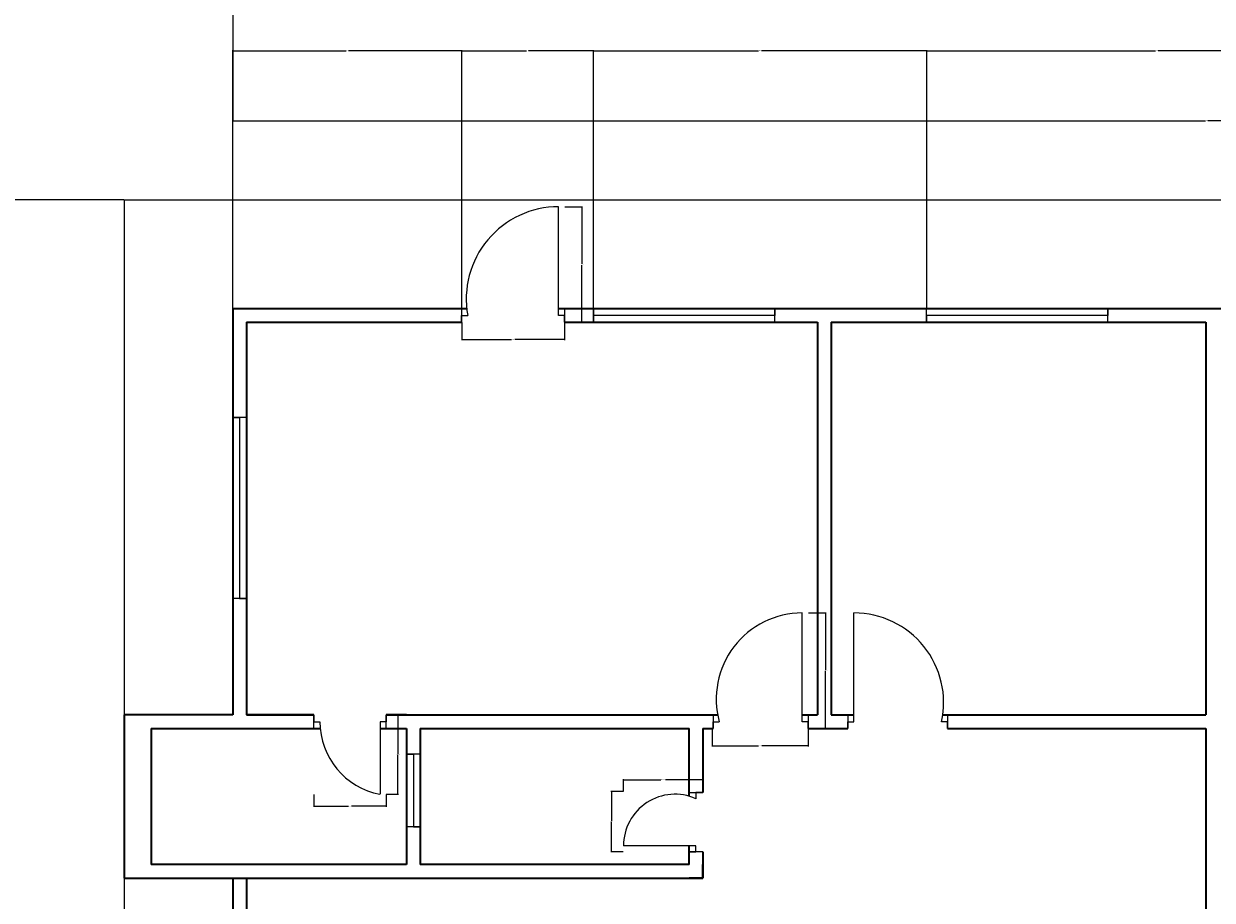
# Model space of a CAD drawing. Units: inches. Extents: x 1520 to 3401, y 1570 to 3432.
# Tile 12 of 15: x 2435 to 2828, y 2501 to 2791. Entities that reach past the tile are written whole.
import ezdxf

# ---------------------------------------------------------------- set-up
doc = ezdxf.new("R2010")
doc.units = ezdxf.units.IN
for name, color, linetype, lineweight in [('A-ANNO-DIMS', 2, 'Continuous', 18), ('A-DOOR', 3, 'Continuous', 18), ('A-FLOR-EDGE', 7, 'Continuous', 25), ('A-GLAZ', 4, 'Continuous', 18), ('A-WALL', 7, 'Continuous', 35)]:
    doc.layers.add(name, color=color, linetype=linetype, lineweight=lineweight)
doc.styles.get("Standard").update_dxf_attribs({"font": 'arial.ttf'})
doc.dimstyles.get("Standard").update_dxf_attribs({"dimtxt": 0.18, "dimasz": 0.18, "dimexe": 0.18, "dimexo": 0.0625, "dimgap": 0.09, "dimtad": 0, "dimtih": 1, "dimtoh": 1, "dimdec": 4, "dimzin": 0, "dimdsep": 46, "dimtxsty": 'Standard', "dimcen": 0.09, "dimadec": 0, "dimazin": 0, "dimtfac": 1, "dimtdec": 4, "dimtofl": 0, "dimtmove": 0, "dimatfit": 3, "dimfxl": 1, "dimtolj": 1, "dimtzin": 0, "dimarcsym": 0})

# ---------------------------------------------------------------- blocks, each defined once
blk = doc.blocks.new('DOOR-SWING-24-01')
for p, q in [((21.75, 19.61), (26.25, 19.61)), ((26.25, 19.61), (24, 19.61)), ((24, 19.61), (24, 17.61)), ((24, 2), (0, 2)), ((24, 0), (24, 2)), ((26.25, 0), (21.75, 0)), ((21.75, 0), (24, 0))]:
    blk.add_line(p, q)
blk.add_arc((17.08, 2), 17.08, 66.0978, 180)
blk = doc.blocks.new('DOOR-SWING-24-02')
for p, q in [((0, 21.75), (0, 26.25)), ((0, 26.25), (0, 24)), ((0, 24), (2, 24)), ((23.89, 24), (21.89, 24)), ((21.89, 24), (21.89, 0)), ((23.89, 21.75), (23.89, 26.25)), ((23.89, 26.25), (23.89, 24))]:
    blk.add_line(p, q)
blk.add_arc((26.42, 24), 24.42, 180, 259.3013)
blk = doc.blocks.new('DOOR-SWING-36-03')
for p, q in [((29.45, 2.25), (29.45, 38.25)), ((0, 4.5), (0, 0)), ((31.45, 4.5), (31.45, 0)), ((0, 0), (0, 2.25)), ((0, 2.25), (2, 2.25)), ((31.45, 2.25), (29.45, 2.25)), ((31.45, 0), (31.45, 2.25))]:
    blk.add_line(p, q)
blk.add_arc((29.45, 9.79), 28.46, 90, 195.3561)
blk = doc.blocks.new('DOOR-SWING-36-04')
for p, q in [((2, 2.25), (2, 38.25)), ((0, 4.5), (0, 0)), ((32.99, 4.5), (32.99, 0)), ((0, 0), (0, 2.25)), ((0, 2.25), (2, 2.25)), ((32.99, 2.25), (30.99, 2.25)), ((32.99, 0), (32.99, 2.25))]:
    blk.add_line(p, q)
blk.add_arc((2, 8.58), 29.67, 347.6919, 90)
blk = doc.blocks.new('DOOR-SWING-36-22')
for p, q in [((32.08, 2.25), (32.08, 38.25)), ((0, 4.5), (0, 0)), ((34.08, 4.5), (34.08, 0)), ((0, 0), (0, 2.25)), ((0, 2.25), (2, 2.25)), ((34.08, 2.25), (32.08, 2.25)), ((34.08, 0), (34.08, 2.25))]:
    blk.add_line(p, q)
blk.add_arc((32.08, 7.69), 30.56, 90, 190.2449)
blk = doc.blocks.new('WIN-PLAN-24-01')
for p, q in [((0, 4.5), (0, 0)), ((24, 2.25), (24, 4.5)), ((24, 4.5), (24, 0)), ((0, 0), (0, 2.25)), ((0, 2.25), (24, 2.25))]:
    blk.add_line(p, q)
blk = doc.blocks.new('WIN-PLAN-60-02')
for p, q in [((4.5, 60), (0, 60)), ((0, 60), (2.25, 60)), ((2.25, 60), (2.25, 0)), ((4.5, 0), (0, 0)), ((2.25, 0), (4.5, 0))]:
    blk.add_line(p, q)
blk = doc.blocks.new('WIN-PLAN-60-03')
for p, q in [((0, 2.25), (0, 4.5)), ((0, 4.5), (0, 0)), ((60, 0), (60, 4.5)), ((60, 4.5), (60, 2.25)), ((60, 2.25), (0, 2.25))]:
    blk.add_line(p, q)
blk = doc.blocks.new('*D81')
at = {"layer": 'A-ANNO-DIMS', "color": 0, "lineweight": -2, "transparency": 16777216}
for p, q in [((2633.15, 2537.36), (2633.15, 2541.41)), ((2633.33, 2541.23), (2645.48, 2541.23)), ((2659.22, 2541.23), (2647.06, 2541.23)), ((2659.4, 2537.36), (2659.4, 2541.41))]:
    blk.add_line(p, q, dxfattribs=at)
at = {"layer": 'A-ANNO-DIMS', "color": 0, "transparency": 16777216}
for points in [[(2633.33, 2541.26), (2633.33, 2541.2), (2633.15, 2541.23)], [(2659.22, 2541.26), (2659.22, 2541.2), (2659.4, 2541.23)]]:
    blk.add_solid(points, dxfattribs=at)
at = {"layer": 'Defpoints', "color": 0, "transparency": 16777216}
for p in [(2659.4, 2541.23), (2633.15, 2537.3), (2659.4, 2537.3)]:
    blk.add_point(p, dxfattribs=at)
at = {"layer": 'A-ANNO-DIMS', "color": 0, "transparency": 16777216, "insert": (2646.27, 2541.23), "char_height": 0.18, "attachment_point": 5}
blk.add_mtext('\\A1;D01 26 TYP.', dxfattribs=at)
blk = doc.blocks.new('*D82')
at = {"layer": 'A-ANNO-DIMS', "color": 0, "lineweight": -2, "transparency": 16777216}
for p, q in [((2633.09, 2537.3), (2629.03, 2537.3)), ((2629.21, 2537.12), (2629.21, 2527.5)), ((2629.21, 2517.52), (2629.21, 2527.14)), ((2633.09, 2517.34), (2629.03, 2517.34))]:
    blk.add_line(p, q, dxfattribs=at)
at = {"layer": 'A-ANNO-DIMS', "color": 0, "transparency": 16777216}
for points in [[(2629.18, 2537.12), (2629.24, 2537.12), (2629.21, 2537.3)], [(2629.18, 2517.52), (2629.24, 2517.52), (2629.21, 2517.34)]]:
    blk.add_solid(points, dxfattribs=at)
at = {"layer": 'Defpoints', "color": 0, "transparency": 16777216}
for p in [(2629.21, 2537.3), (2633.15, 2537.3), (2633.15, 2517.34)]:
    blk.add_point(p, dxfattribs=at)
at = {"layer": 'A-ANNO-DIMS', "color": 0, "transparency": 16777216, "insert": (2629.21, 2527.32), "char_height": 0.18, "attachment_point": 5}
blk.add_mtext('\\A1;20 TYP.', dxfattribs=at)
blk = doc.blocks.new('*D83')
at = {"layer": 'A-ANNO-DIMS', "color": 0, "lineweight": -2, "transparency": 16777216}
for p, q in [((2554.66, 2562.68), (2558.71, 2562.68)), ((2558.53, 2562.5), (2558.53, 2549.74)), ((2558.53, 2536.61), (2558.53, 2549.37)), ((2554.66, 2536.43), (2558.71, 2536.43))]:
    blk.add_line(p, q, dxfattribs=at)
at = {"layer": 'A-ANNO-DIMS', "color": 0, "transparency": 16777216}
for points in [[(2558.5, 2562.5), (2558.56, 2562.5), (2558.53, 2562.68)], [(2558.5, 2536.61), (2558.56, 2536.61), (2558.53, 2536.43)]]:
    blk.add_solid(points, dxfattribs=at)
at = {"layer": 'Defpoints', "color": 0, "transparency": 16777216}
for p in [(2554.6, 2562.68), (2558.53, 2562.68), (2554.6, 2536.43)]:
    blk.add_point(p, dxfattribs=at)
at = {"layer": 'A-ANNO-DIMS', "color": 0, "transparency": 16777216, "insert": (2558.53, 2549.55), "char_height": 0.18, "attachment_point": 5}
blk.add_mtext('\\A1;D02 26 TYP.', dxfattribs=at)
blk = doc.blocks.new('*D84')
at = {"layer": 'A-ANNO-DIMS', "color": 0, "lineweight": -2, "transparency": 16777216}
for p, q in [((2530.7, 2536.37), (2530.7, 2532.31)), ((2554.6, 2536.37), (2554.6, 2532.31)), ((2530.88, 2532.49), (2542.12, 2532.49)), ((2554.42, 2532.49), (2543.18, 2532.49))]:
    blk.add_line(p, q, dxfattribs=at)
at = {"layer": 'A-ANNO-DIMS', "color": 0, "transparency": 16777216}
for points in [[(2530.88, 2532.52), (2530.88, 2532.46), (2530.7, 2532.49)], [(2554.42, 2532.52), (2554.42, 2532.46), (2554.6, 2532.49)]]:
    blk.add_solid(points, dxfattribs=at)
at = {"layer": 'Defpoints', "color": 0, "transparency": 16777216}
for p in [(2530.7, 2536.43), (2554.6, 2536.43), (2554.6, 2532.49)]:
    blk.add_point(p, dxfattribs=at)
at = {"layer": 'A-ANNO-DIMS', "color": 0, "transparency": 16777216, "insert": (2542.65, 2532.49), "char_height": 0.18, "attachment_point": 5}
blk.add_mtext('\\A1;24 TYP.', dxfattribs=at)
blk = doc.blocks.new('*D85')
at = {"layer": 'A-ANNO-DIMS', "color": 0, "lineweight": -2, "transparency": 16777216}
for p, q in [((2694.38, 2596.43), (2700.24, 2596.43)), ((2700.06, 2596.25), (2700.06, 2577.49)), ((2700.06, 2558.36), (2700.06, 2577.12)), ((2694.38, 2558.18), (2700.24, 2558.18))]:
    blk.add_line(p, q, dxfattribs=at)
at = {"layer": 'A-ANNO-DIMS', "color": 0, "transparency": 16777216}
for points in [[(2700.03, 2596.25), (2700.09, 2596.25), (2700.06, 2596.43)], [(2700.03, 2558.36), (2700.09, 2558.36), (2700.06, 2558.18)]]:
    blk.add_solid(points, dxfattribs=at)
at = {"layer": 'Defpoints', "color": 0, "transparency": 16777216}
for p in [(2694.32, 2596.43), (2700.06, 2596.43), (2694.32, 2558.18)]:
    blk.add_point(p, dxfattribs=at)
at = {"layer": 'A-ANNO-DIMS', "color": 0, "transparency": 16777216, "insert": (2700.06, 2577.3), "char_height": 0.18, "attachment_point": 5}
blk.add_mtext('\\A1;D03 38 TYP.', dxfattribs=at)
blk = doc.blocks.new('*D86')
at = {"layer": 'A-ANNO-DIMS', "color": 0, "lineweight": -2, "transparency": 16777216}
for p, q in [((2662.52, 2558.12), (2662.52, 2552.26)), ((2694.32, 2558.12), (2694.32, 2552.26)), ((2662.7, 2552.44), (2677.89, 2552.44)), ((2694.14, 2552.44), (2678.95, 2552.44))]:
    blk.add_line(p, q, dxfattribs=at)
at = {"layer": 'A-ANNO-DIMS', "color": 0, "transparency": 16777216}
for points in [[(2662.7, 2552.47), (2662.7, 2552.41), (2662.52, 2552.44)], [(2694.14, 2552.47), (2694.14, 2552.41), (2694.32, 2552.44)]]:
    blk.add_solid(points, dxfattribs=at)
at = {"layer": 'Defpoints', "color": 0, "transparency": 16777216}
for p in [(2662.52, 2558.18), (2694.32, 2558.18), (2694.32, 2552.44)]:
    blk.add_point(p, dxfattribs=at)
at = {"layer": 'A-ANNO-DIMS', "color": 0, "transparency": 16777216, "insert": (2678.42, 2552.44), "char_height": 0.18, "attachment_point": 5}
blk.add_mtext('\\A1;32 TYP.', dxfattribs=at)
blk = doc.blocks.new('*D123')
at = {"layer": 'A-ANNO-DIMS', "color": 0, "lineweight": -2, "transparency": 16777216}
for p, q in [((2613.76, 2730.93), (2619.61, 2730.93)), ((2619.43, 2730.75), (2619.43, 2711.99)), ((2619.43, 2692.86), (2619.43, 2711.62)), ((2613.76, 2692.68), (2619.61, 2692.68))]:
    blk.add_line(p, q, dxfattribs=at)
at = {"layer": 'A-ANNO-DIMS', "color": 0, "transparency": 16777216}
for points in [[(2619.4, 2730.75), (2619.46, 2730.75), (2619.43, 2730.93)], [(2619.4, 2692.86), (2619.46, 2692.86), (2619.43, 2692.68)]]:
    blk.add_solid(points, dxfattribs=at)
at = {"layer": 'Defpoints', "color": 0, "transparency": 16777216}
for p in [(2613.69, 2730.93), (2619.43, 2730.93), (2613.69, 2692.68)]:
    blk.add_point(p, dxfattribs=at)
at = {"layer": 'A-ANNO-DIMS', "color": 0, "transparency": 16777216, "insert": (2619.43, 2711.8), "char_height": 0.18, "attachment_point": 5}
blk.add_mtext('\\A1;D22 38 TYP.', dxfattribs=at)
blk = doc.blocks.new('*D124')
at = {"layer": 'A-ANNO-DIMS', "color": 0, "lineweight": -2, "transparency": 16777216}
for p, q in [((2579.62, 2692.62), (2579.62, 2686.76)), ((2613.69, 2692.62), (2613.69, 2686.76)), ((2579.8, 2686.94), (2596.13, 2686.94)), ((2613.51, 2686.94), (2597.18, 2686.94))]:
    blk.add_line(p, q, dxfattribs=at)
at = {"layer": 'A-ANNO-DIMS', "color": 0, "transparency": 16777216}
for points in [[(2579.8, 2686.97), (2579.8, 2686.91), (2579.62, 2686.94)], [(2613.51, 2686.97), (2613.51, 2686.91), (2613.69, 2686.94)]]:
    blk.add_solid(points, dxfattribs=at)
at = {"layer": 'Defpoints', "color": 0, "transparency": 16777216}
for p in [(2579.62, 2692.68), (2613.69, 2692.68), (2613.69, 2686.94)]:
    blk.add_point(p, dxfattribs=at)
at = {"layer": 'A-ANNO-DIMS', "color": 0, "transparency": 16777216, "insert": (2596.65, 2686.94), "char_height": 0.18, "attachment_point": 5}
blk.add_mtext('\\A1;34 TYP.', dxfattribs=at)
blk = doc.blocks.new('*D192')
at = {"layer": 'A-ANNO-DIMS', "color": 0, "lineweight": -2, "transparency": 16777216}
for p, q in [((2467.84, 2733.18), (2386.32, 2733.18)), ((2386.5, 2733), (2386.5, 2244.61)), ((2386.5, 1755.86), (2386.5, 2244.25)), ((2503.84, 1755.68), (2386.32, 1755.68))]:
    blk.add_line(p, q, dxfattribs=at)
at = {"layer": 'A-ANNO-DIMS', "color": 0, "transparency": 16777216}
for points in [[(2386.47, 2733), (2386.53, 2733), (2386.5, 2733.18)], [(2386.47, 1755.86), (2386.53, 1755.86), (2386.5, 1755.68)]]:
    blk.add_solid(points, dxfattribs=at)
at = {"layer": 'Defpoints', "color": 0, "transparency": 16777216}
for p in [(2467.9, 2733.18), (2386.5, 1755.68), (2503.9, 1755.68)]:
    blk.add_point(p, dxfattribs=at)
at = {"layer": 'A-ANNO-DIMS', "color": 0, "transparency": 16777216, "insert": (2386.5, 2244.43), "char_height": 0.18, "attachment_point": 5}
blk.add_mtext('\\A1;977.5', dxfattribs=at)
blk = doc.blocks.new('*D202')
at = {"layer": 'A-ANNO-DIMS', "color": 0, "lineweight": -2, "transparency": 16777216}
for p, q in [((2503.9, 2697.24), (2503.9, 2782.76)), ((2504.08, 2782.58), (2541.37, 2782.58)), ((2579.44, 2782.58), (2542.15, 2782.58)), ((2579.62, 2692.74), (2579.62, 2782.76))]:
    blk.add_line(p, q, dxfattribs=at)
at = {"layer": 'A-ANNO-DIMS', "color": 0, "transparency": 16777216}
for points in [[(2504.08, 2782.61), (2504.08, 2782.55), (2503.9, 2782.58)], [(2579.44, 2782.61), (2579.44, 2782.55), (2579.62, 2782.58)]]:
    blk.add_solid(points, dxfattribs=at)
at = {"layer": 'Defpoints', "color": 0, "transparency": 16777216}
for p in [(2579.62, 2782.58), (2503.9, 2697.18), (2579.62, 2692.68)]:
    blk.add_point(p, dxfattribs=at)
at = {"layer": 'A-ANNO-DIMS', "color": 0, "transparency": 16777216, "insert": (2541.76, 2782.58), "char_height": 0.18, "attachment_point": 5}
blk.add_mtext('\\A1;75.72', dxfattribs=at)
blk = doc.blocks.new('*D203')
at = {"layer": 'A-ANNO-DIMS', "color": 0, "lineweight": -2, "transparency": 16777216}
for p, q in [((2579.62, 2692.74), (2579.62, 2782.76)), ((2579.8, 2782.58), (2601.09, 2782.58)), ((2623.04, 2782.58), (2601.74, 2782.58)), ((2623.22, 2692.74), (2623.22, 2782.76))]:
    blk.add_line(p, q, dxfattribs=at)
at = {"layer": 'A-ANNO-DIMS', "color": 0, "transparency": 16777216}
for points in [[(2579.8, 2782.61), (2579.8, 2782.55), (2579.62, 2782.58)], [(2623.04, 2782.61), (2623.04, 2782.55), (2623.22, 2782.58)]]:
    blk.add_solid(points, dxfattribs=at)
at = {"layer": 'Defpoints', "color": 0, "transparency": 16777216}
for p in [(2623.22, 2782.58), (2579.62, 2692.68), (2623.22, 2692.68)]:
    blk.add_point(p, dxfattribs=at)
at = {"layer": 'A-ANNO-DIMS', "color": 0, "transparency": 16777216, "insert": (2601.42, 2782.58), "char_height": 0.18, "attachment_point": 5}
blk.add_mtext('\\A1;43.6', dxfattribs=at)
blk = doc.blocks.new('*D204')
at = {"layer": 'A-ANNO-DIMS', "color": 0, "lineweight": -2, "transparency": 16777216}
for p, q in [((2623.22, 2692.74), (2623.22, 2782.76)), ((2623.4, 2782.58), (2677.9, 2782.58)), ((2733.32, 2782.58), (2678.81, 2782.58)), ((2733.5, 2697.24), (2733.5, 2782.76))]:
    blk.add_line(p, q, dxfattribs=at)
at = {"layer": 'A-ANNO-DIMS', "color": 0, "transparency": 16777216}
for points in [[(2623.4, 2782.61), (2623.4, 2782.55), (2623.22, 2782.58)], [(2733.32, 2782.61), (2733.32, 2782.55), (2733.5, 2782.58)]]:
    blk.add_solid(points, dxfattribs=at)
at = {"layer": 'Defpoints', "color": 0, "transparency": 16777216}
for p in [(2733.5, 2782.58), (2733.5, 2697.18), (2623.22, 2692.68)]:
    blk.add_point(p, dxfattribs=at)
at = {"layer": 'A-ANNO-DIMS', "color": 0, "transparency": 16777216, "insert": (2678.36, 2782.58), "char_height": 0.18, "attachment_point": 5}
blk.add_mtext('\\A1;110.28', dxfattribs=at)
blk = doc.blocks.new('*D205')
at = {"layer": 'A-ANNO-DIMS', "color": 0, "lineweight": -2, "transparency": 16777216}
for p, q in [((2733.5, 2697.24), (2733.5, 2782.76)), ((2733.68, 2782.58), (2809.22, 2782.58)), ((2885.68, 2782.58), (2810.13, 2782.58)), ((2885.86, 2692.74), (2885.86, 2782.76))]:
    blk.add_line(p, q, dxfattribs=at)
at = {"layer": 'A-ANNO-DIMS', "color": 0, "transparency": 16777216}
for points in [[(2733.68, 2782.61), (2733.68, 2782.55), (2733.5, 2782.58)], [(2885.68, 2782.61), (2885.68, 2782.55), (2885.86, 2782.58)]]:
    blk.add_solid(points, dxfattribs=at)
at = {"layer": 'Defpoints', "color": 0, "transparency": 16777216}
for p in [(2885.86, 2782.58), (2733.5, 2697.18), (2885.86, 2692.68)]:
    blk.add_point(p, dxfattribs=at)
at = {"layer": 'A-ANNO-DIMS', "color": 0, "transparency": 16777216, "insert": (2809.68, 2782.58), "char_height": 0.18, "attachment_point": 5}
blk.add_mtext('\\A1;152.37', dxfattribs=at)
blk = doc.blocks.new('*D224')
at = {"layer": 'A-ANNO-DIMS', "color": 0, "lineweight": -2, "transparency": 16777216}
for p, q in [((2503.9, 2875.57), (2503.9, 2759.2)), ((3148.4, 2875.57), (3148.4, 2759.2)), ((2504.08, 2759.38), (2825.75, 2759.38)), ((3148.22, 2759.38), (2826.54, 2759.38))]:
    blk.add_line(p, q, dxfattribs=at)
at = {"layer": 'A-ANNO-DIMS', "color": 0, "transparency": 16777216}
for points in [[(2504.08, 2759.41), (2504.08, 2759.35), (2503.9, 2759.38)], [(3148.22, 2759.41), (3148.22, 2759.35), (3148.4, 2759.38)]]:
    blk.add_solid(points, dxfattribs=at)
at = {"layer": 'Defpoints', "color": 0, "transparency": 16777216}
for p in [(2503.9, 2875.63), (3148.4, 2875.63), (3148.4, 2759.38)]:
    blk.add_point(p, dxfattribs=at)
at = {"layer": 'A-ANNO-DIMS', "color": 0, "transparency": 16777216, "insert": (2826.15, 2759.38), "char_height": 0.18, "attachment_point": 5}
blk.add_mtext('\\A1;644.5', dxfattribs=at)

msp = doc.modelspace()

# ---------------------------------------------------------------- linework, layer by layer
at = {"layer": 'A-FLOR-EDGE'}
for q in [(2467.8987, 1791.6786), (3184.3987, 2733.1786)]:
    msp.add_line((2467.8987, 2733.1786), q, dxfattribs=at)
at = {"layer": 'A-WALL'}
for p, q in [((2503.8987, 2697.1786), (2503.8987, 2562.6786)), ((2503.8987, 2697.1786), (2503.8987, 2562.6786)), ((2503.8987, 2697.1786), (2581.2953, 2697.1786)), ((2611.6928, 2697.1786), (2887.6429, 2697.1786)), ((2508.3987, 2692.6786), (2508.3987, 2562.6786)), ((2508.3987, 2692.6786), (2579.616, 2692.6786)), ((2613.6928, 2692.6786), (2697.3987, 2692.6786)), ((2697.3987, 2692.6786), (2697.3987, 2562.6786)), ((2701.8987, 2692.6786), (2701.8987, 2562.6786)), ((2701.8987, 2692.6786), (2825.8987, 2692.6786)), ((2825.8987, 2692.6786), (2825.8987, 2562.6786)), ((2503.8987, 2562.6786), (2467.8987, 2562.6786)), ((2467.8987, 2562.6786), (2467.8987, 2508.6786)), ((2508.3987, 2562.6786), (2530.705, 2562.6786)), ((2530.705, 2562.6786), (2508.3987, 2562.6786)), ((2554.5952, 2562.6786), (2664.3512, 2562.6786)), ((2561.3987, 2562.6786), (2554.5952, 2562.6786)), ((2692.3184, 2562.6786), (2697.3987, 2562.6786)), ((2701.8987, 2562.6786), (2709.4502, 2562.6786)), ((2738.8433, 2562.6786), (2825.8987, 2562.6786)), ((2476.8987, 2558.1786), (2532.8088, 2558.1786)), ((2476.8987, 2558.1786), (2476.8987, 2513.1786)), ((2552.5952, 2558.1786), (2561.3987, 2558.1786)), ((2561.3987, 2558.1786), (2561.3987, 2513.1786)), ((2565.8987, 2558.1786), (2565.8987, 2513.1786)), ((2565.8987, 2558.1786), (2654.8987, 2558.1786)), ((2654.8987, 2535.7697), (2654.8987, 2558.1786)), ((2659.3987, 2558.1786), (2662.8719, 2558.1786)), ((2659.3987, 2558.1786), (2659.3987, 2536.9559)), ((2694.3184, 2558.1786), (2707.4502, 2558.1786)), ((2740.4425, 2558.1786), (2825.8987, 2558.1786)), ((2825.8987, 2558.1786), (2825.8987, 2343.1786)), ((2654.8987, 2513.1786), (2654.8987, 2519.341)), ((2659.3987, 2517.341), (2659.3987, 2508.6786)), ((2561.3987, 2513.1786), (2476.8987, 2513.1786)), ((2654.8987, 2513.1786), (2565.8987, 2513.1786)), ((2659.3987, 2508.6786), (2659.3987, 2513.1786)), ((2467.8987, 2508.6786), (2565.8987, 2508.6786)), ((2503.8987, 2508.6786), (2503.8987, 2425.0977)), ((2503.8987, 2508.6786), (2503.8987, 2425.0977)), ((2508.3987, 2508.6786), (2508.3987, 2423.0977)), ((2508.3987, 2508.6786), (2631.3987, 2508.6786)), ((2565.8987, 2508.6786), (2631.3987, 2508.6786)), ((2631.3987, 2508.6786), (2635.8987, 2508.6786)), ((2635.8987, 2508.6786), (2654.8987, 2508.6786)), ((2659.3987, 2508.6786), (2654.8987, 2508.6786)), ((2654.8987, 2508.6786), (2659.3987, 2508.6786))]:
    msp.add_line(p, q, dxfattribs=at)

# ---------------------------------------------------------------- block references
at = {"layer": 'A-DOOR'}
for name, p in [('DOOR-SWING-36-22', (2579.6158, 2692.679)), ('DOOR-SWING-36-03', (2662.8718, 2558.179)), ('DOOR-SWING-36-04', (2707.4498, 2558.179)), ('DOOR-SWING-24-02', (2530.7048, 2536.429)), ('DOOR-SWING-24-01', (2633.1488, 2517.341))]:
    msp.add_blockref(name, p, dxfattribs=at)
at = {"layer": 'A-GLAZ'}
for name, p in [('WIN-PLAN-60-03', (2623.2164, 2692.679)), ('WIN-PLAN-60-02', (2503.8988, 2601.185))]:
    msp.add_blockref(name, p, dxfattribs=at)
at = {"layer": 'A-GLAZ', "rotation": 270}
for name, p in [('WIN-PLAN-60-02', (2733.496, 2697.1785)), ('WIN-PLAN-24-01', (2561.399, 2549.6622))]:
    msp.add_blockref(name, p, dxfattribs=at)

# ---------------------------------------------------------------- dimensions: what is measured, and where the dimension line sits
at = {"layer": 'A-ANNO-DIMS'}
for base, p1, p2, override, picture, middle in [((3148.3987, 2759.3805), (2503.8987, 2875.633), (3148.3987, 2875.633), {"dimdec": 1, "dimlfac": 1, "dimrnd": 0, "dimzin": 0, "dimdsep": 46, "dimlunit": 2}, '*D224', (2826.1487, 2759.3805)), ((2579.616, 2782.5786), (2503.8987, 2697.1786), (2579.616, 2692.6786), {"dimdec": 2, "dimlfac": 1, "dimrnd": 0, "dimzin": 0, "dimdsep": 46, "dimlunit": 2}, '*D202', (2541.7573, 2782.5786)), ((2623.2166, 2782.5786), (2579.616, 2692.6786), (2623.2166, 2692.6786), {"dimdec": 1, "dimlfac": 1, "dimrnd": 0, "dimzin": 0, "dimdsep": 46, "dimlunit": 2}, '*D203', (2601.4163, 2782.5786)), ((2733.4955, 2782.5786), (2623.2166, 2692.6786), (2733.4955, 2697.1786), {"dimdec": 2, "dimlfac": 1, "dimrnd": 0, "dimzin": 0, "dimdsep": 46, "dimlunit": 2}, '*D204', (2678.3561, 2782.5786)), ((2885.8633, 2782.5786), (2733.4955, 2697.1786), (2885.8633, 2692.6786), {"dimdec": 2, "dimlfac": 1, "dimrnd": 0, "dimzin": 0, "dimdsep": 46, "dimlunit": 2}, '*D205', (2809.6794, 2782.5786))]:
    dim = msp.add_linear_dim(base=base, p1=p1, p2=p2, dimstyle='Standard', override=override, dxfattribs=at)
    dim.commit()
    dim.dimension.update_dxf_attribs({"geometry": picture, "text_midpoint": middle})
dim = msp.add_linear_dim(base=(2386.4982, 1755.6786), p1=(2467.8987, 2733.1786), p2=(2503.8987, 1755.6786), angle=90, dimstyle='Standard', override={"dimdec": 1, "dimlfac": 1, "dimrnd": 0, "dimzin": 0, "dimdsep": 46, "dimlunit": 2}, dxfattribs=at)
dim.commit()
dim.dimension.update_dxf_attribs({"geometry": '*D192', "text_midpoint": (2386.4982, 2244.4286)})
for base, p1, p2, text, picture, middle in [((2619.4303, 2730.9286), (2613.6928, 2692.6786), (2613.6928, 2730.9286), 'D22 <> TYP.', '*D123', (2619.4303, 2711.8036)), ((2700.0559, 2596.4286), (2694.3184, 2558.1786), (2694.3184, 2596.4286), 'D03 <> TYP.', '*D85', (2700.0559, 2577.3036)), ((2558.5327, 2562.6786), (2554.5952, 2536.4286), (2554.5952, 2562.6786), 'D02 <> TYP.', '*D83', (2558.5327, 2549.5536)), ((2629.2112, 2537.2972), (2633.1487, 2517.341), (2633.1487, 2537.2972), '<> TYP.', '*D82', (2629.2112, 2527.3191))]:
    dim = msp.add_linear_dim(base=base, p1=p1, p2=p2, angle=90, text=text, dimstyle='Standard', override={"dimdec": 0, "dimlfac": 1, "dimrnd": 0, "dimzin": 0, "dimdsep": 46, "dimlunit": 2}, dxfattribs=at)
    dim.commit()
    dim.dimension.update_dxf_attribs({"geometry": picture, "text_midpoint": middle})
for base, p1, p2, text, picture, middle in [((2613.6928, 2686.9411), (2579.616, 2692.6786), (2613.6928, 2692.6786), '<> TYP.', '*D124', (2596.6544, 2686.9411)), ((2694.3184, 2552.4411), (2662.5204, 2558.1786), (2694.3184, 2558.1786), '<> TYP.', '*D86', (2678.4194, 2552.4411)), ((2659.3987, 2541.2347), (2633.1487, 2537.2972), (2659.3987, 2537.2972), 'D01 <> TYP.', '*D81', (2646.2737, 2541.2347)), ((2554.5952, 2532.4911), (2530.705, 2536.4286), (2554.5952, 2536.4286), '<> TYP.', '*D84', (2542.6501, 2532.4911))]:
    dim = msp.add_linear_dim(base=base, p1=p1, p2=p2, text=text, dimstyle='Standard', override={"dimdec": 0, "dimlfac": 1, "dimrnd": 0, "dimzin": 0, "dimdsep": 46, "dimlunit": 2}, dxfattribs=at)
    dim.commit()
    dim.dimension.update_dxf_attribs({"geometry": picture, "text_midpoint": middle})

doc.saveas('drawing.dxf')
